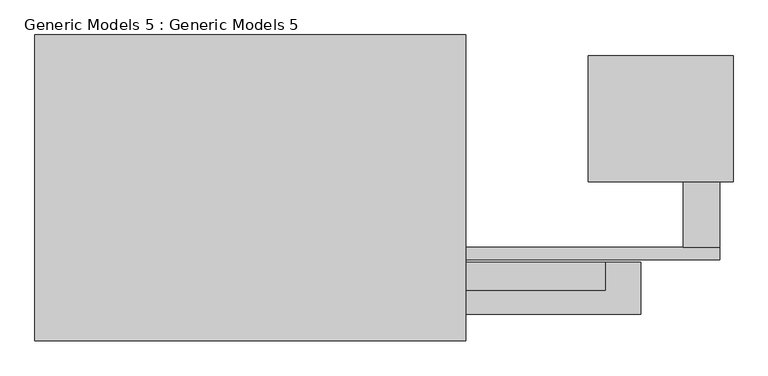
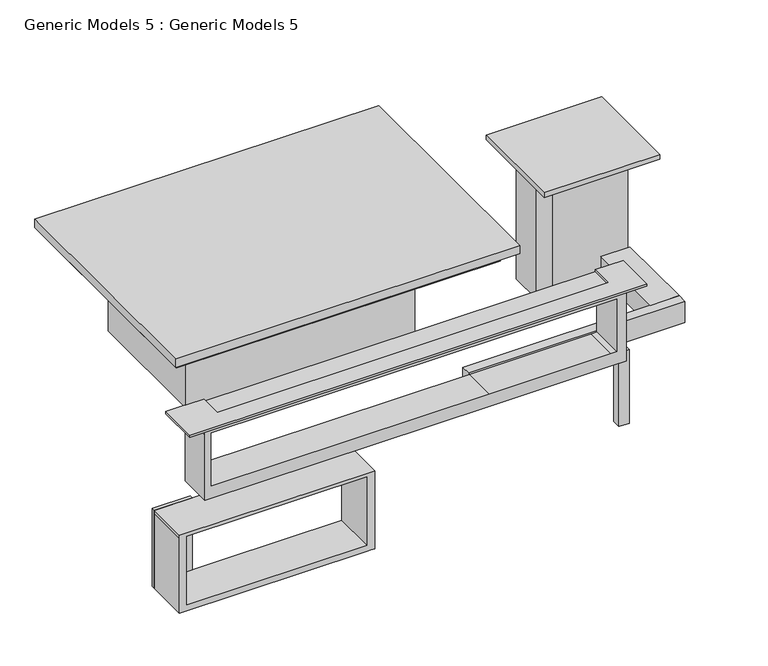
"""IFC4 building model written with IfcOpenShell, lengths in millimetres: proxy geometry, Generic Models 5 : Generic Models 5."""

from ifc_helpers import new_model, si_unit, frame, origin, origin_with_axes, place, context, project, spatial, polyline, outline, extrude, faceted_brep, source, transform, mapped, element, save


def generic_models_5_generic_models_5_34eadfb7(model_context):
    return source(origin(), model_context, "Body", "SolidModel", [
        extrude(outline(polyline([(-18801.416554, -12309.2493389), (-18801.416554, -10853.2015118), (-17472.2745558, -10853.2015118), (-17472.2745558, -11656.7266818), (-3734.5414835, -11656.7266818), (-3734.5414835, -10853.2015118), (-2759.3020237, -10853.2015118), (-2759.3020237, -12309.2493389), (-18801.416554, -12309.2493389)])), frame((0.0, 0.0, 6400.8), z_axis=(0.0, 0.0, 1.0), x_axis=(1.0, 0.0, 0.0)), (0.0, 0.0, 1.0), 76.2),
        faceted_brep([(-18126.3020237, -10853.2015118, 6400.8), (-18126.3020237, -6166.9015118, 6400.8), (-10068.0026327, -6166.9015118, 6400.8), (-10068.0026327, -10853.2015118, 6400.8), (-10068.0026327, -10853.2015118, 9475.9806962), (-18126.3020237, -10853.2015118, 9475.9806962), (-10068.0026327, -6166.9015118, 9475.9806962), (-18126.3020237, -6166.9015118, 9475.9806962), (-19516.8026327, -5133.8524785, 9780.7806962), (-19516.8026327, -12720.1015118, 9780.7806962), (-8144.1020237, -12720.1015118, 9780.7806962), (-8144.1020237, -5133.8524785, 9780.7806962), (-19516.8026327, -5133.8524785, 9475.9806962), (-8144.1020237, -5133.8524785, 9475.9806962), (-8144.1020237, -12720.1015118, 9475.9806962), (-19516.8026327, -12720.1015118, 9475.9806962)], [[[0, 1, 2, 3]], [[0, 3, 4, 5]], [[3, 2, 6, 4]], [[2, 1, 7, 6]], [[1, 0, 5, 7]], [[8, 9, 10, 11]], [[12, 13, 14, 15], [5, 4, 6, 7]], [[9, 8, 12, 15]], [[10, 9, 15, 14]], [[11, 10, 14, 13]], [[8, 11, 13, 12]]]),
        faceted_brep([(-610.0530902, -5501.0544656, 3352.8), (-610.0530902, -7432.5524785, 3352.8), (-3267.3020237, -7432.5524785, 3352.8), (-3826.1020237, -7432.5524785, 3352.8), (-3826.1020237, -6217.7015118, 3352.8), (-3267.3020237, -6217.7015118, 3352.8), (-3267.3020237, -5501.0544656, 3352.8), (-3267.3020237, -5501.0544656, 7965.1861127), (-610.0530902, -5501.0544656, 7965.1861127), (-3267.3020237, -6217.7015118, 7965.1861127), (-3826.1020237, -6217.7015118, 7965.1861127), (-3826.1020237, -7432.5524785, 7965.1861127), (-3267.3020237, -7432.5524785, 7965.1861127), (-610.0530902, -7432.5524785, 7965.1861127), (-168.5020237, -8602.0582153, 8136.4223222), (-168.5020237, -5070.3524785, 8136.4223222), (-4227.9399536, -5070.3524785, 8136.4223222), (-4227.9399536, -8602.0582153, 8136.4223222), (-168.5020237, -8602.0582153, 7965.1861127), (-4227.9399536, -8602.0582153, 7965.1861127), (-4227.9399536, -5070.3524785, 7965.1861127), (-168.5020237, -5070.3524785, 7965.1861127)], [[[0, 1, 2, 3, 4, 5, 6]], [[0, 6, 7, 8]], [[6, 5, 9, 7]], [[5, 4, 10, 9]], [[4, 3, 11, 10]], [[3, 2, 12, 11]], [[2, 1, 13, 12]], [[1, 0, 8, 13]], [[14, 15, 16, 17]], [[18, 19, 20, 21], [8, 7, 9, 10, 11, 12, 13]], [[15, 14, 18, 21]], [[16, 15, 21, 20]], [[17, 16, 20, 19]], [[14, 17, 19, 18]]]),
        extrude(outline(polyline([(2767.5752588, -19167.7020237), (0.0, -19167.7020237), (0.0, -12596.0998458), (0.0, -12462.1020237), (0.0, -12309.7020237), (2894.5752588, -12309.7020237), (2894.5752588, -19167.7020237), (2767.5752588, -19167.7020237)]), holes=[polyline([(227.5752588, -12596.0998458), (227.5752588, -18920.6998458), (2767.5752588, -18920.6998458), (2767.5752588, -12596.0998458), (227.5752588, -12596.0998458)])]), frame((0.0, -12309.2493389, 0.0), z_axis=(0.0, 1.0, 0.0), x_axis=(0.0, 0.0, 1.0)), (0.0, 0.0, 1.0), 1519.5478271),
        extrude(outline(polyline([(-19167.7020237, -10789.7015118), (-19167.7020237, -10662.7015118), (-17842.4229687, -10662.7015118), (-17842.4229687, -10789.7015118), (-19167.7020237, -10789.7015118)])), origin_with_axes(), (0.0, 0.0, 1.0), 2894.5752588),
        extrude(outline(polyline([(-2505.3020237, -10789.7015118), (-2868.5085537, -10789.7015118), (-2868.5085537, -10484.9015118), (-2505.3020237, -10484.9015118), (-2505.3020237, -10789.7015118)])), frame((0.0, 0.0, 304.8), z_axis=(0.0, 0.0, 1.0), x_axis=(1.0, 0.0, 0.0)), (0.0, 0.0, 1.0), 2743.2),
        extrude(outline(polyline([(-19726.5020237, -4488.4302839), (-7657.5286199, -4488.4302839), (-7657.5286199, -13058.6524785), (-19726.5020237, -13058.6524785), (-19726.5020237, -4488.4302839)])), frame((0.0, 0.0, 9780.7806962), z_axis=(0.0, 0.0, 1.0), x_axis=(1.0, 0.0, 0.0)), (0.0, 0.0, 1.0), 304.8),
        extrude(outline(polyline([(-546.7793301, -10434.1015118), (-1562.7793301, -10434.1015118), (-1562.7793301, -7436.9015118), (-546.7793301, -7436.9015118), (-546.7793301, -10434.1015118)])), frame((0.0, 0.0, 3352.8), z_axis=(0.0, 0.0, 1.0), x_axis=(1.0, 0.0, 0.0)), (0.0, 0.0, 1.0), 782.7328571),
        extrude(outline(polyline([(6400.8, -18126.3020237), (6096.0, -18126.3020237), (3673.6016483, -18126.3020237), (3673.6016483, -8144.1020237), (3673.6016483, -3876.9020237), (3673.6016483, -3343.5020237), (6400.8, -3343.5020237), (6400.8, -18126.3020237)]), holes=[polyline([(4135.5328571, -17897.7020237), (6096.0, -17897.7020237), (6096.0, -3673.7020237), (4135.5328571, -3673.7020237), (4135.5328571, -3876.9020237), (4135.5328571, -8144.1020237), (4135.5328571, -17897.7020237)])]), frame((0.0, -12051.1125482, 0.0), z_axis=(0.0, 1.0, 0.0), x_axis=(0.0, 0.0, 1.0)), (0.0, 0.0, 1.0), 1197.9110364),
        extrude(outline(polyline([(-546.7793301, -10789.7015118), (-8144.1020237, -10789.7015118), (-8144.1020237, -10434.1015118), (-546.7793301, -10434.1015118), (-546.7793301, -10789.7015118)])), frame((0.0, 0.0, 3352.8), z_axis=(0.0, 0.0, 1.0), x_axis=(1.0, 0.0, 0.0)), (0.0, 0.0, 1.0), 782.7328571),
    ])


if __name__ == "__main__":
    model = new_model("IFC4")
    model_context = context("Model", 3, world=origin())
    ifc_project = project(units=[si_unit("LENGTHUNIT", "METRE", prefix="MILLI")], contexts=[model_context])
    site = spatial("IfcSite", under=ifc_project)
    building = spatial("IfcBuilding", under=site)
    placement = place(None, origin())
    generic_models_5_generic_models_5_shape = generic_models_5_generic_models_5_34eadfb7(model_context)
    element("IfcBuildingElementProxy", 1, Name="Generic Models 5 : Generic Models 5", ObjectType="Generic Models 5 : Generic Models 5", at=placement, inside=building, context=model_context, shape_type="MappedRepresentation", body=[
        mapped(generic_models_5_generic_models_5_shape, transform((0.0, 0.0, 0.0), x_axis=(1.0, 0.0, 0.0), y_axis=(0.0, 1.0, 0.0), z_axis=(0.0, 0.0, 1.0))),
    ])
    save(model, "model.ifc")

# Revit data of these elements
# Element 1 (IfcBuildingElementProxy, "Generic Models 5 : Generic Models 5")
#   Materials on its faces: "Tile, Mosaic, Gray", "Tile, Porcelain, 4in"
# Materials
#   "Tile, Mosaic, Gray": class "Generic", colour RGB 127 127 127, transparency 0, Description = "Mosiac tile, gray", Cost = 0
#   "Tile, Porcelain, 4in": class "Generic", colour RGB 89 87 158, transparency 0, Description = "Porcelain tile, 4\", white", Cost = 0
